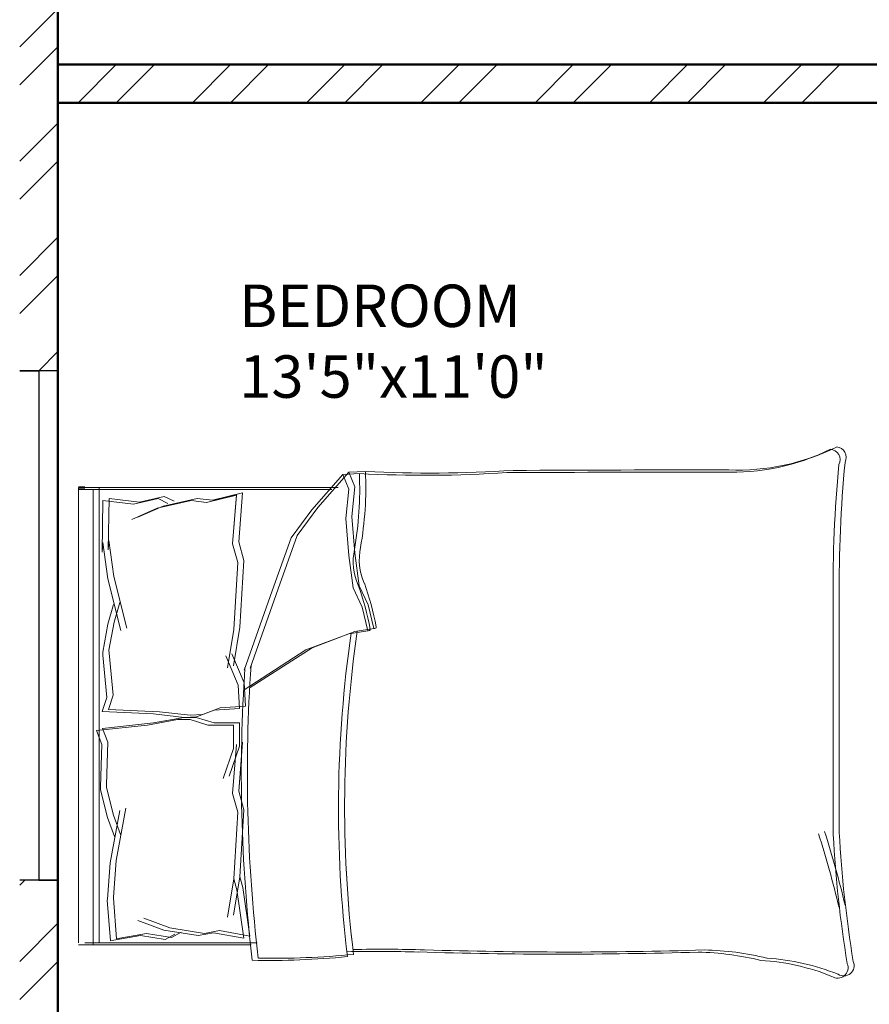
# Model space of a CAD drawing. Units: inches. Extents: x 1901 to 2863, y 888 to 2433.
# Tile 24 of 91: x 2439 to 2540, y 1289 to 1405. Entities that reach past the tile are written whole.
import ezdxf

# ---------------------------------------------------------------- set-up
doc = ezdxf.new("R2010")
doc.units = ezdxf.units.IN
for name, color, linetype, lineweight in [('A-AREA-IDEN', 7, 'Continuous', 18), ('A-FURN', 8, 'Continuous', 18), ('A-GLAZ', 3, 'Continuous', 25), ('A-WALL', 7, 'Continuous', 50), ('A-WALL-PATT', 8, 'Continuous', 13)]:
    doc.layers.add(name, color=color, linetype=linetype, lineweight=lineweight)
doc.styles.get("Standard").update_dxf_attribs({"font": 'arial.ttf'})

# ---------------------------------------------------------------- blocks, each defined once
blk = doc.blocks.new('BED-DOUBLE')
for p, q in [((31.18, 59.32), (27.53, 55.16)), ((31.18, 59.32), (27.53, 55.16)), ((31.9, 59.58), (28.25, 55.42)), ((31.9, 59.58), (28.25, 55.42)), ((33.14, 59.41), (31.18, 59.32, 4.35)), ((33.14, 59.41), (31.18, 59.32, 4.35)), ((31.87, 57.59), (31.18, 59.32)), ((31.87, 57.59), (31.18, 59.32)), ((33.85, 59.67), (31.9, 59.58, 4.35)), ((33.85, 59.67), (31.9, 59.58, 4.35)), ((32.59, 57.85), (31.9, 59.58)), ((32.59, 57.85), (31.9, 59.58)), ((0.03, 57.78), (0.03, 4.12)), ((0.74, 57.78), (30.62, 57.78)), ((0.74, 57.78), (30.62, 57.78)), ((18.63, 56.89), (15.11, 56.01)), ((18.63, 56.88), (15.11, 56.01)), ((19.35, 57.14), (15.83, 56.27)), ((19.35, 57.14), (15.83, 56.27)), ((18.18, 51.12), (18.63, 56.89)), ((18.18, 51.12), (18.63, 56.88)), ((18.9, 51.38), (19.35, 57.14)), ((18.9, 51.38), (19.35, 57.14)), ((31.53, 54.12), (31.87, 57.59)), ((31.53, 54.12), (31.87, 57.59)), ((32.24, 54.37), (32.59, 57.85)), ((32.24, 54.37), (32.59, 57.85)), ((2.9, 56.23), (2.79, 50.16)), ((2.9, 56.23), (2.79, 50.16)), ((2.9, 56.23), (6.5, 55.8)), ((2.9, 56.23), (6.5, 55.8)), ((3.61, 56.48), (3.51, 50.42)), ((3.61, 56.48), (3.51, 50.42)), ((3.61, 56.48), (7.22, 56.06)), ((3.61, 56.48), (7.22, 56.06)), ((6.5, 55.8), (9.39, 56.47)), ((6.5, 55.8), (9.39, 56.47)), ((7.22, 56.06), (10.11, 56.73)), ((7.22, 56.06), (10.11, 56.73)), ((13.31, 56.23), (9.3, 55.33)), ((13.31, 56.23), (9.3, 55.33)), ((9.39, 56.47), (10.56, 55.89)), ((9.39, 56.47), (10.56, 55.89)), ((14.02, 56.48), (10.01, 55.58)), ((14.02, 56.48), (10.01, 55.58)), ((10.11, 56.73), (11.28, 56.15)), ((10.11, 56.73), (11.28, 56.15)), ((15.11, 56.01), (13.31, 56.23)), ((15.11, 56.01), (13.31, 56.23)), ((15.83, 56.27), (14.02, 56.48)), ((15.83, 56.27), (14.02, 56.48)), ((9.3, 55.33), (6.29, 54)), ((9.3, 55.33), (6.29, 54)), ((10.01, 55.58), (7.01, 54.26)), ((10.01, 55.58), (7.01, 54.26)), ((27.53, 55.16), (25.1, 51.86)), ((27.53, 55.16), (25.1, 51.86)), ((28.25, 55.42), (25.81, 52.11)), ((28.25, 55.42), (25.81, 52.11)), ((31.87, 49.77), (31.53, 54.12)), ((31.87, 49.77), (31.53, 54.12)), ((32.59, 50.03), (32.24, 54.37)), ((32.59, 50.03), (32.24, 54.37)), ((2.79, 50.16), (2.88, 51.29)), ((2.79, 50.16), (2.88, 51.29)), ((2.88, 51.29), (3.47, 47.02)), ((2.88, 51.29), (3.47, 47.02)), ((3.51, 50.42), (3.6, 51.54)), ((3.51, 50.42), (3.6, 51.54)), ((3.6, 51.54), (4.19, 47.28)), ((3.6, 51.54), (4.19, 47.28)), ((18.81, 48.92), (18.18, 51.12)), ((18.81, 48.92), (18.18, 51.12)), ((19.52, 49.18), (18.9, 51.38)), ((19.52, 49.18), (18.9, 51.38)), ((25.1, 51.86), (22.84, 45.6)), ((25.1, 51.86), (22.84, 45.6)), ((25.81, 52.11), (23.55, 45.85)), ((25.81, 52.11), (23.55, 45.85)), ((33.11, 46.2), (32.59, 50.03)), ((33.11, 46.2), (32.59, 50.03)), ((18.32, 41.05), (18.81, 48.92)), ((18.32, 41.05), (18.81, 48.92)), ((19.04, 41.31), (19.52, 49.18)), ((19.04, 41.31), (19.52, 49.18)), ((32.39, 45.94), (31.87, 49.77)), ((32.39, 45.94), (31.87, 49.77)), ((3.47, 47.02), (4.99, 40.94)), ((3.47, 47.02), (4.99, 40.94)), ((4.19, 47.28), (5.71, 41.19)), ((4.19, 47.28), (5.71, 41.19)), ((22.84, 45.6), (19.54, 36.24)), ((22.84, 45.6), (19.54, 36.24)), ((23.55, 45.85), (20.26, 36.49)), ((23.55, 45.85), (20.26, 36.49)), ((33.44, 43.68), (32.39, 45.94)), ((33.44, 43.68), (32.39, 45.94)), ((34.15, 43.94), (33.11, 46.2)), ((34.15, 43.94), (33.11, 46.2)), ((4.87, 44.23), (4.2, 41.91)), ((4.87, 44.23), (4.2, 41.91)), ((89, 16.88), (89, 44.51)), ((89, 16.88), (89, 44.51)), ((89.72, 17.13), (89.72, 44.77)), ((89.72, 17.13), (89.72, 44.77)), ((4.15, 43.98), (3.48, 41.66)), ((4.15, 43.98), (3.48, 41.66)), ((34.13, 40.9), (33.44, 43.68)), ((34.13, 40.9), (33.44, 43.68)), ((34.85, 41.16), (34.15, 43.94)), ((34.85, 41.16), (34.15, 43.94)), ((4.2, 41.91), (3.59, 38.62)), ((4.2, 41.91), (3.59, 38.62)), ((3.48, 41.66), (2.87, 38.37)), ((3.48, 41.66), (2.87, 38.37)), ((17.57, 36.53), (18.32, 41.05)), ((17.57, 36.52), (18.32, 41.05)), ((18.29, 36.78), (19.04, 41.31)), ((18.29, 36.78), (19.04, 41.31)), ((27.55, 38.9), (32.59, 40.81)), ((27.55, 38.9), (32.59, 40.81)), ((31.87, 40.55), (34.13, 40.9)), ((31.87, 40.55), (34.13, 40.9)), ((32.59, 40.81), (34.85, 41.16)), ((32.59, 40.81), (34.85, 41.16)), ((26.83, 38.64), (31.87, 40.55)), ((26.83, 38.64), (31.87, 40.55)), ((2.87, 38.37), (2.9, 38.01)), ((2.87, 38.37), (2.9, 38.01)), ((3.59, 38.62), (3.62, 38.26)), ((3.59, 38.62), (3.62, 38.26)), ((19.54, 33.94), (26.83, 38.64)), ((19.54, 33.94), (26.83, 38.64)), ((20.26, 34.19), (27.55, 38.9)), ((20.26, 34.19), (27.55, 38.9)), ((2.9, 38.01), (3.37, 33.03)), ((2.9, 38.01), (3.37, 33.04)), ((3.62, 38.26), (4.09, 33.29)), ((3.62, 38.26), (4.09, 33.29)), ((18.82, 34.49), (17.38, 37.94)), ((18.82, 34.49), (17.38, 37.94)), ((19.54, 34.74), (18.1, 38.19)), ((19.54, 34.74), (18.1, 38.19)), ((18.99, 31.73), (18.82, 34.49)), ((18.99, 31.73), (18.82, 34.49)), ((19.71, 31.99), (19.54, 34.74)), ((19.71, 31.99), (19.54, 34.74)), ((3.37, 33.04), (2.82, 31.37)), ((3.37, 33.03), (2.82, 31.37)), ((4.09, 33.29), (3.54, 31.63)), ((4.09, 33.29), (3.54, 31.63)), ((2.82, 31.37), (8.86, 31.1)), ((2.82, 31.37), (8.86, 31.1)), ((3.54, 31.63), (9.58, 31.36)), ((3.54, 31.63), (9.58, 31.36)), ((9.58, 31.36), (13.18, 30.93)), ((9.58, 31.36), (13.18, 30.93)), ((13.92, 30.77), (15.99, 31.55)), ((13.92, 30.77), (15.99, 31.55)), ((14.64, 31.02), (16.71, 31.8)), ((14.64, 31.02), (16.71, 31.8)), ((15.99, 31.55), (18.99, 31.73)), ((15.99, 31.55), (18.99, 31.73)), ((16.71, 31.8), (19.71, 31.99)), ((16.71, 31.8), (19.71, 31.99)), ((8.13, 29.78), (11.7, 30.43)), ((8.13, 29.78), (11.7, 30.43)), ((8.85, 30.04), (12.42, 30.69)), ((8.85, 30.04), (12.42, 30.69)), ((8.86, 31.1), (12.46, 30.68)), ((8.86, 31.1), (12.46, 30.68)), ((11.7, 30.43), (13.16, 30.43)), ((11.7, 30.43), (13.16, 30.43)), ((12.42, 30.69), (13.88, 30.69)), ((12.42, 30.69), (13.88, 30.69)), ((12.46, 30.68), (13.92, 30.77)), ((12.46, 30.68), (13.92, 30.77)), ((13.16, 30.43), (15.28, 29.78)), ((13.16, 30.43), (15.28, 29.78)), ((13.18, 30.93), (14.64, 31.02)), ((13.18, 30.93), (14.64, 31.02)), ((13.88, 30.69), (15.99, 30.04)), ((13.88, 30.69), (15.99, 30.04)), ((2.13, 29.14), (8.13, 29.78)), ((2.13, 29.14), (8.13, 29.78)), ((2.78, 27.51), (2.13, 29.14)), ((2.78, 27.51), (2.13, 29.14)), ((2.84, 29.39), (8.85, 30.04)), ((2.84, 29.39), (8.85, 30.04)), ((3.49, 27.77), (2.84, 29.39)), ((3.49, 27.77), (2.84, 29.39)), ((15.28, 29.78), (18.29, 29.78)), ((15.28, 29.78), (18.29, 29.78)), ((15.99, 30.04), (19, 30.04)), ((15.99, 30.04), (19, 30.04)), ((18.29, 29.78), (18.29, 27.03)), ((18.29, 29.78), (18.29, 27.03)), ((19, 30.04), (19, 27.28)), ((19, 30.04), (19, 27.28)), ((2.61, 22.52), (2.78, 27.51)), ((2.61, 22.52), (2.78, 27.51)), ((3.33, 22.78), (3.49, 27.77)), ((3.33, 22.78), (3.49, 27.77)), ((18.29, 27.03), (17.06, 23.49)), ((18.29, 27.03), (17.06, 23.5)), ((19, 27.28), (17.78, 23.75)), ((19, 27.28), (17.78, 23.75)), ((18.18, 21.73), (18.63, 27.49)), ((18.18, 21.73), (18.63, 27.49)), ((18.9, 21.98), (19.35, 27.75)), ((18.9, 21.98), (19.35, 27.74)), ((2.61, 22.16), (2.61, 22.52)), ((2.61, 22.16), (2.61, 22.52)), ((3.42, 18.91), (2.61, 22.16)), ((3.42, 18.91), (2.61, 22.16)), ((3.33, 22.42), (3.33, 22.78)), ((3.33, 22.42), (3.33, 22.78)), ((4.14, 19.17), (3.33, 22.42)), ((4.14, 19.17), (3.33, 22.42)), ((18.81, 19.53), (18.18, 21.73)), ((18.81, 19.53), (18.18, 21.73)), ((19.52, 19.78), (18.9, 21.98)), ((19.52, 19.78), (18.9, 21.98)), ((3.75, 13.56), (4.89, 19.73)), ((3.75, 13.56), (4.89, 19.73)), ((4.47, 13.81), (5.6, 19.98)), ((4.47, 13.81), (5.6, 19.98)), ((19.04, 11.91), (19.52, 19.78)), ((19.04, 11.91), (19.52, 19.78)), ((4.24, 16.64), (3.42, 18.91)), ((4.24, 16.64), (3.42, 18.91)), ((4.95, 16.9), (4.14, 19.17)), ((4.95, 16.9), (4.14, 19.17)), ((18.32, 11.66), (18.81, 19.53)), ((18.32, 11.66), (18.81, 19.53)), ((3.42, 9.27), (3.75, 13.56)), ((3.42, 9.27), (3.75, 13.56)), ((4.14, 9.52), (4.47, 13.81)), ((4.14, 9.52), (4.47, 13.81)), ((17.57, 7.13), (18.32, 11.66)), ((17.57, 7.13), (18.32, 11.66)), ((18.29, 7.38), (19.04, 11.91)), ((18.29, 7.39), (19.04, 11.91)), ((18.32, 11.66), (18.68, 10.38)), ((18.32, 11.66), (18.68, 10.38)), ((19.04, 11.91), (19.4, 10.64)), ((19.04, 11.91), (19.4, 10.64)), ((19.4, 10.64), (20.21, 4.92)), ((19.4, 10.64), (20.21, 4.92)), ((4.12, 9.4), (4.14, 9.52)), ((4.12, 9.4), (4.14, 9.52)), ((4.49, 4.6), (4.12, 9.4)), ((4.49, 4.6), (4.12, 9.4)), ((18.68, 10.38), (19.5, 4.66)), ((18.68, 10.38), (19.5, 4.66)), ((3.4, 9.15), (3.42, 9.27)), ((3.4, 9.15), (3.42, 9.27)), ((3.77, 4.34), (3.4, 9.15)), ((3.77, 4.34), (3.4, 9.15)), ((10.8, 5.89), (7.71, 7.03)), ((10.8, 5.89), (7.71, 7.03)), ((10.08, 5.63), (7, 6.77)), ((10.08, 5.63), (7, 6.77)), ((14.86, 5.24), (10.8, 5.89)), ((14.86, 5.24), (10.8, 5.89)), ((3.75, 4.34), (7.32, 4.99)), ((3.75, 4.34), (7.32, 4.99)), ((4.47, 4.59), (8.04, 5.24)), ((4.47, 4.59), (8.04, 5.24)), ((7.32, 4.99), (10.24, 4.5)), ((7.32, 4.99), (10.24, 4.5)), ((8.04, 5.24), (10.96, 4.75)), ((8.04, 5.24), (10.96, 4.76)), ((14.14, 4.99), (10.08, 5.63)), ((14.14, 4.99), (10.08, 5.63)), ((10.24, 4.5), (11.38, 5.15)), ((10.24, 4.5), (11.38, 5.15)), ((10.96, 4.76), (12.1, 5.4)), ((10.96, 4.75), (12.1, 5.4)), ((15.92, 5.31), (14.14, 4.99)), ((15.92, 5.31), (14.14, 4.99)), ((16.64, 5.57), (14.86, 5.24)), ((16.64, 5.57), (14.86, 5.24)), ((19.5, 4.66), (15.92, 5.31)), ((19.5, 4.66), (15.92, 5.31)), ((20.21, 4.92), (16.64, 5.57)), ((20.21, 4.92), (16.64, 5.57))]:
    blk.add_line(p, q)
for centre, radius, start, end in [((77.12, 85.47), 25.9, 267.4714, 296.4681), ((77.12, 85.47), 25.9, 267.4714, 296.4681), ((77.84, 85.73), 25.9, 267.4714, 296.4681), ((77.84, 85.73), 25.9, 267.4714, 296.4681), ((88.58, 61.05), 1.24, 332.6588, 86.02), ((88.58, 61.05), 1.24, 332.6588, 86.02), ((89.3, 61.31), 1.24, 332.6588, 86.02), ((89.3, 61.31), 1.24, 332.6588, 86.02), ((238.36, 46.17), 149.37, 174.4998, 180.6351), ((238.36, 46.17), 149.37, 174.4998, 180.6351), ((239.08, 46.42), 149.37, 174.4998, 180.6351), ((239.08, 46.42), 149.37, 174.4998, 180.6351), ((-7.45, 57.59), 40.62, 349.8763, 2.5657), ((-7.45, 57.59), 40.62, 349.8763, 2.5657), ((40.8, 204.6), 145.39, 266.9791, 273.8365), ((40.8, 204.6), 145.39, 266.9791, 273.8365), ((-6.73, 57.85), 40.62, 349.8763, 2.5657), ((-6.73, 57.85), 40.62, 349.8763, 2.5657), ((41.52, 204.86), 145.39, 266.9791, 273.8365), ((41.52, 204.86), 145.39, 266.9791, 273.8365), ((76.17, -5062.23), 5121.82, 90.00217, 90.28689), ((76.17, -5062.23), 5121.82, 90.00217, 90.28689), ((76.89, -5061.97), 5121.82, 90.00217, 90.28689), ((76.89, -5061.97), 5121.82, 90.00217, 90.28689), ((39.4, 49.08), 6.99, 168.6608, 203.7384), ((39.4, 49.08), 6.99, 168.6608, 203.7384), ((40.11, 49.33), 6.99, 168.6608, 203.7384), ((40.11, 49.33), 6.99, 168.6608, 203.7384), ((2.41, 35.2), 33.29, 10.6617, 19.8806), ((2.41, 35.2), 33.29, 10.6617, 19.8806), ((1.69, 34.94), 33.29, 10.6617, 19.8806), ((1.69, 34.94), 33.29, 10.6617, 19.8806), ((176.25, 20.16), 144.86, 171.7845, 186.9006), ((176.25, 20.15), 144.86, 171.7845, 186.9006), ((34.2, 41.1), 0.207, 250.2464, 1.1377), ((34.2, 41.1), 0.207, 250.2464, 1.1377), ((34.92, 41.35), 0.207, 250.2464, 1.1377), ((34.92, 41.35), 0.207, 250.2464, 1.1377), ((175.53, 19.9), 144.86, 171.7845, 186.9006), ((175.53, 19.9), 144.86, 171.7845, 186.9006), ((204.43, 23.94), 185.22, 176.0865, 186.7821), ((204.43, 23.94), 185.22, 176.0865, 186.7821), ((205.14, 24.2), 185.22, 176.0865, 186.7821), ((205.14, 24.2), 185.22, 176.0865, 186.7821), ((225.52, 24.02), 136.7, 182.9958, 189.4091), ((225.52, 24.02), 136.7, 182.9958, 189.4091), ((226.23, 24.28), 136.7, 182.9958, 189.4091), ((226.23, 24.28), 136.7, 182.9958, 189.4091), ((22.59, 95.58), 93.53, 268.7218, 275.604), ((22.59, 95.58), 93.53, 268.7218, 275.604), ((23.31, 95.84), 93.53, 268.7218, 275.604), ((23.31, 95.84), 93.53, 268.7218, 275.604), ((35.03, -187.88), 190.99, 88.4762, 91.0082), ((35.03, -187.88), 190.99, 88.4762, 91.0082), ((35.74, -187.62), 190.99, 88.4762, 91.0082), ((35.74, -187.62), 190.99, 88.4762, 91.0082), ((56.85, 544.3), 541.51, 268.2277, 271.7185), ((56.85, 544.3), 541.51, 268.2277, 271.7185), ((57.57, 544.55), 541.51, 268.2277, 271.7185), ((57.57, 544.55), 541.51, 268.2277, 271.7185), ((72.46, -30.24), 33.27, 76.0648, 88.9113), ((72.46, -30.24), 33.27, 76.0648, 88.9113), ((73.18, -29.98), 33.27, 76.0648, 88.9113), ((73.18, -29.98), 33.27, 76.0648, 88.9113), ((78.93, -24.35), 26.45, 67.9751, 86.652), ((78.93, -24.35), 26.45, 67.9751, 86.652), ((79.65, -24.1), 26.45, 67.9751, 86.652), ((79.65, -24.1), 26.45, 67.9751, 86.652), ((89.53, 1.18), 1.22, 236.1736, 23.4781), ((89.53, 1.18), 1.22, 236.1736, 23.4781), ((90.25, 1.44), 1.22, 236.1736, 23.4781), ((90.25, 1.44), 1.22, 236.1736, 23.4781)]:
    blk.add_arc(centre, radius, start, end)
blk = doc.blocks.new('WIN-60')
for p, q in [((0, 4.5), (0, 0)), ((60, 2.25), (60, 4.5)), ((60, 4.5), (60, 0)), ((0, 0), (0, 2.25)), ((0, 2.25), (60, 2.25))]:
    blk.add_line(p, q)

msp = doc.modelspace()

# ---------------------------------------------------------------- hatches: boundary and pattern name
at = {"layer": 'A-WALL-PATT'}
h = msp.add_hatch(dxfattribs=at)
h.set_pattern_fill('ANSI32', color=256)
h.paths.add_polyline_path([(2192.5, 2274.13), (2141.26, 2274.13), (2141.26, 2269.63), (2192.5, 2269.63)])
h.paths.add_polyline_path([(2259.93, 2274.13), (2216.5, 2274.13), (2216.5, 2269.63), (2255.43, 2269.63), (2255.43, 2214.63), (2250.81, 2214.63), (2250.81, 2210.13), (2259.93, 2210.13), (2259.93, 2215.13), (2271.76, 2215.13), (2271.76, 2217.38), (2271.76, 2219.63), (2259.93, 2219.63)])
h.paths.add_polyline_path([(2171.43, 2269.63), (2166.93, 2269.63), (2166.93, 2219.63), (2121.24, 2219.63), (2121.24, 2215.13), (2166.93, 2215.13), (2166.93, 2083.13), (2161.81, 2083.13), (2161.81, 2078.63), (2171.43, 2078.63), (2177, 2078.63), (2177, 2080.88), (2177, 2083.13), (2171.43, 2083.13), (2171.43, 2210.13), (2230.91, 2210.13), (2230.91, 2212.38), (2230.91, 2214.63), (2171.43, 2214.63)])
h.paths.add_polyline_path([(2117.26, 2274.13), (2089.43, 2274.13), (2089.43, 2219.63), (2081.14, 2219.63), (2081.14, 2215.13), (2089.43, 2215.13), (2098, 2215.13), (2098, 2217.38), (2098, 2219.63), (2093.93, 2219.63), (2093.93, 2269.63), (2117.26, 2269.63), (2117.26, 2271.88)])
h.paths.add_polyline_path([(2343.43, 2219.63), (2329.29, 2219.63), (2329.29, 2215.13), (2338.93, 2215.13), (2338.93, 2184.74), (2343.43, 2184.74)])
h.paths.add_polyline_path([(2338.93, 2083.13), (2329.29, 2083.13), (2208.97, 2083.13), (2208.97, 2078.63), (2338.93, 2078.63)])
h.paths.add_polyline_path([(2343.43, 2136.74), (2338.93, 2136.74), (2338.93, 1872.63), (2343.43, 1872.63)])
h.paths.add_polyline_path([(2343.43, 1863.63), (2397.68, 1863.63), (2397.68, 1821.63), (2384.14, 1821.63), (2384.14, 1812.63), (2418.33, 1812.63), (2418.33, 1817.13), (2418.33, 1821.63), (2406.68, 1821.63), (2406.68, 1863.63), (2459.5, 1863.63), (2459.5, 1821.63), (2447.14, 1821.63), (2447.14, 1812.63), (2459.5, 1812.63), (2468.5, 1812.63), (2468.5, 1872.63), (2394.43, 1872.63), (2334.43, 1872.63), (2334.43, 1812.63), (2343.43, 1812.63), (2353.25, 1812.63), (2353.25, 1821.63), (2343.43, 1821.63)])
h.paths.add_polyline_path([(2510.01, 1872.63), (2468.5, 1872.63), (2468.5, 1868.13), (2510.01, 1868.13)])
h.paths.add_polyline_path([(2514.01, 1817.13), (2468.5, 1817.13), (2468.5, 1812.63), (2482.11, 1812.63), (2482.11, 1800.61), (2486.61, 1800.61), (2486.61, 1812.63), (2514.01, 1812.63)])
h.paths.add_polyline_path([(2299.25, 1814.88), (2299.25, 1817.13), (2295.93, 1817.13), (2295.93, 1854.17), (2293.68, 1854.17), (2291.43, 1854.17), (2291.43, 1817.13), (2266.11, 1817.13), (2266.11, 1812.63), (2299.25, 1812.63)])
h.paths.add_polyline_path([(2218.11, 1817.13), (2206.46, 1817.13), (2171.43, 1817.13), (2171.43, 1949.13), (2190.1, 1949.13), (2190.1, 1953.63), (2163.47, 1953.63), (2163.47, 1949.13), (2166.93, 1949.13), (2166.93, 1817.13), (2114.3, 1817.13), (2114.3, 1812.63), (2218.11, 1812.63)])
h.paths.add_polyline_path([(2029.43, 1970.92), (2024.93, 1970.92), (2024.93, 1912.72), (2029.43, 1912.72)])
h.paths.add_polyline_path([(2132.3, 1953.63), (2113.93, 1953.63), (2113.93, 1975.89), (2111.68, 1975.89), (2109.43, 1975.89), (2109.43, 1953.63), (2029.43, 1953.63), (2029.43, 1949.13), (2132.3, 1949.13)])
h.paths.add_polyline_path([(2029.43, 1853.61), (2029.31, 1853.61), (2029.31, 1853.61), (2029.43, 1853.61), (2029.43, 1864.72), (2024.93, 1864.72), (2024.93, 1812.63), (2066.3, 1812.63), (2066.3, 1814.88), (2066.3, 1817.13), (2029.43, 1817.13)])
h.paths.add_polyline_path([(2122.93, 2010.09), (2120.68, 2010.09), (2118.43, 2010.09), (2118.43, 2006.13), (2029.43, 2006.13), (2029.43, 2001.63), (2109.43, 2001.63), (2109.43, 1998.04), (2113.93, 1998.04), (2113.93, 2001.63), (2122.93, 2001.63)])
h.paths.add_polyline_path([(2029.43, 2031.38), (2024.93, 2031.38), (2024.93, 1994.92), (2027.18, 1994.92), (2029.43, 1994.92)])
h.paths.add_polyline_path([(2029.43, 2136.74), (2024.93, 2136.74), (2024.93, 2067.38), (2027.18, 2067.38), (2029.43, 2067.38)])
h.paths.add_polyline_path([(2125.62, 2083.13), (2029.43, 2083.13), (2029.43, 2078.63), (2118.43, 2078.63), (2118.43, 2030.71), (2122.93, 2030.71), (2122.93, 2078.63), (2125.62, 2078.63)])
h.paths.add_polyline_path([(2029.43, 2215.13), (2040.47, 2215.13), (2040.47, 2217.38), (2040.47, 2219.63), (2024.93, 2219.63), (2024.93, 2184.74), (2029.43, 2184.74), (2029.43, 2187.78)])
h.paths.add_polyline_path([(2686.43, 2274.13), (2659.28, 2274.13), (2659.28, 2269.63), (2681.93, 2269.63), (2681.93, 2219.63), (2676.82, 2219.63), (2676.82, 2215.13), (2681.93, 2215.13), (2697.01, 2215.13), (2697.01, 2217.38), (2697.01, 2219.63), (2686.43, 2219.63)])
h.paths.add_polyline_path([(2609.93, 2269.63), (2635.28, 2269.63), (2635.28, 2274.13), (2571.43, 2274.13), (2571.43, 2269.63), (2605.43, 2269.63), (2605.43, 2214.63), (2549.1, 2214.63), (2549.1, 2210.13), (2605.43, 2210.13), (2605.43, 2083.13), (2601.01, 2083.13), (2601.01, 2080.88), (2601.01, 2078.63), (2609.93, 2078.63), (2616.16, 2078.63), (2616.16, 2080.88), (2616.16, 2083.13), (2609.93, 2083.13), (2609.93, 2215.13), (2651.46, 2215.13), (2651.46, 2217.38), (2651.46, 2219.63), (2609.93, 2219.63)])
h.paths.add_polyline_path([(2521.43, 2269.63), (2547.43, 2269.63), (2547.43, 2271.88), (2547.43, 2274.13), (2516.93, 2274.13), (2516.93, 2219.63), (2506.41, 2219.63), (2506.41, 2215.13), (2516.93, 2215.13), (2516.93, 2210.13), (2525.4, 2210.13), (2525.4, 2212.38), (2525.4, 2214.63), (2521.43, 2214.63)])
h.paths.add_polyline_path([(2456.01, 2219.63), (2439.43, 2219.63), (2439.43, 2187.89), (2443.93, 2187.89), (2443.93, 2215.13), (2456.01, 2215.13)])
h.paths.add_polyline_path([(2752.93, 2219.63), (2739.48, 2219.63), (2739.48, 2215.13), (2748.43, 2215.13), (2748.43, 2187.89), (2752.93, 2187.89)])
h.paths.add_polyline_path([(2752.93, 2139.89), (2748.43, 2139.89), (2748.43, 2083.13), (2648.42, 2083.13), (2648.42, 2078.63), (2654.93, 2078.63), (2654.93, 2039.44), (2659.43, 2039.44), (2659.43, 2078.63), (2748.43, 2078.63), (2748.43, 2063.43), (2752.93, 2063.43)])
h.paths.add_polyline_path([(2752.93, 2010.63), (2659.43, 2010.63), (2659.43, 2015.65), (2654.93, 2015.65), (2654.93, 2010.63), (2605.43, 2010.63), (2605.43, 1920.97), (2609.93, 1920.97), (2609.93, 2006.13), (2748.43, 2006.13), (2748.43, 1982.47), (2752.93, 1982.47)])
h.paths.add_polyline_path([(2752.93, 2027.43), (2748.43, 2027.43), (2748.43, 2010.63), (2752.93, 2010.63)])
h.paths.add_polyline_path([(2748.43, 1886.13), (2609.93, 1886.13), (2609.93, 1889.72), (2605.43, 1889.72), (2605.43, 1861.26), (2609.93, 1861.26), (2609.93, 1881.63), (2748.43, 1881.63)])
h.paths.add_polyline_path([(2456.86, 2228.83), (2498.4, 2228.83), (2498.4, 2247.49), (2456.86, 2247.49)], flags=9)
h.paths.add_polyline_path([(2038.6, 2237.42), (2080.17, 2237.42), (2080.17, 2256.08), (2038.6, 2256.08)], flags=9)
h.paths.add_polyline_path([(2292.01, 1062.39), (2539.93, 1062.39), (2539.93, 1099.49), (2292.01, 1099.49)], flags=9)
h.paths.add_polyline_path([(2424.91, 1832.25), (2448.51, 1832.25), (2448.51, 1846.68), (2424.91, 1846.68)], flags=25)
h.paths.add_polyline_path([(2359.08, 1832.25), (2382.68, 1832.25), (2382.68, 1846.68), (2359.08, 1846.68)], flags=25)
h.paths.add_polyline_path([(2352.9, 1684.8), (2367.54, 1684.8), (2367.54, 1697.17), (2352.9, 1697.17)], flags=9)
h.paths.add_polyline_path([(2079.29, 1755.83), (2169.02, 1755.83), (2169.02, 1774.37), (2079.29, 1774.37)], flags=9)
h.paths.add_polyline_path([(2404.09, 1373.86), (2404.09, 1463.59), (2385.54, 1463.59), (2385.54, 1373.86)], flags=9)
h.paths.add_polyline_path([(2268.09, 2236.37), (2309.64, 2236.37), (2309.64, 2255.03), (2268.09, 2255.03)], flags=9)
h.paths.add_polyline_path([(2575.96, 1700.95), (2665.7, 1700.95), (2665.7, 1719.5), (2575.96, 1719.5)], flags=9)
h.paths.add_polyline_path([(2302.96, 1878.47), (2329.52, 1878.47), (2329.52, 1888.78), (2302.96, 1888.78)], flags=9)
h.paths.add_polyline_path([(2097.42, 2240.58), (2126.57, 2240.58), (2126.57, 2259.23), (2097.42, 2259.23)], flags=9)
h.paths.add_polyline_path([(2208.72, 2246.12), (2237.88, 2246.12), (2237.88, 2264.78), (2208.72, 2264.78)], flags=9)
h.paths.add_polyline_path([(2038.15, 1925.96), (2076.99, 1925.96), (2076.99, 1944.62), (2038.15, 1944.62)], flags=9)
h.paths.add_polyline_path([(2239.14, 1926.67), (2288.46, 1926.67), (2288.46, 1945.33), (2239.14, 1945.33)], flags=9)
h.paths.add_polyline_path([(2175.43, 2007.33), (2212.36, 2007.33), (2212.36, 2025.99), (2175.43, 2025.99)], flags=9)
h.paths.add_polyline_path([(2225.03, 2091.79), (2263.87, 2091.79), (2263.87, 2110.45), (2225.03, 2110.45)], flags=9)
h.paths.add_polyline_path([(2035.4, 2098.48), (2074.24, 2098.48), (2074.24, 2117.14), (2035.4, 2117.14)], flags=9)
h.paths.add_polyline_path([(2050.1, 2029.21), (2083.26, 2029.21), (2083.26, 2047.87), (2050.1, 2047.87)], flags=9)
h.paths.add_polyline_path([(2069.68, 1956.72), (2098.83, 1956.72), (2098.83, 1975.38), (2069.68, 1975.38)], flags=25)
h.paths.add_polyline_path([(2328.62, 1753.34), (2361.66, 1753.34), (2361.66, 1771.99), (2328.62, 1771.99)], flags=9)
h.paths.add_polyline_path([(2395.16, 2060.89), (2395.16, 2140.65), (2378.68, 2140.65), (2378.68, 2060.89)], flags=9)
h.paths.add_polyline_path([(2463.73, 2059.02), (2492.89, 2059.02), (2492.89, 2077.68), (2463.73, 2077.68)], flags=9)
h.paths.add_polyline_path([(2458.03, 2181.54), (2496.87, 2181.54), (2496.87, 2200.19), (2458.03, 2200.19)], flags=9)
h.paths.add_polyline_path([(2527.58, 2243.07), (2556.73, 2243.07), (2556.73, 2261.73), (2527.58, 2261.73)], flags=9)
h.paths.add_polyline_path([(2694.46, 2232.77), (2736.03, 2232.77), (2736.03, 2251.42), (2694.46, 2251.42)], flags=9)
h.paths.add_polyline_path([(2637.82, 2249.22), (2666.98, 2249.22), (2666.98, 2267.88), (2637.82, 2267.88)], flags=9)
h.paths.add_polyline_path([(2623.69, 2183.54), (2662.53, 2183.54), (2662.53, 2202.2), (2623.69, 2202.2)], flags=9)
h.paths.add_polyline_path([(2691.97, 2021.5), (2725.12, 2021.5), (2725.12, 2040.16), (2691.97, 2040.16)], flags=9)
h.paths.add_polyline_path([(2621.04, 1975.91), (2662.34, 1975.91), (2662.34, 1994.57), (2621.04, 1994.57)], flags=25)
h.paths.add_polyline_path([(2479.03, 1927.62), (2519.84, 1927.62), (2519.84, 1946.28), (2479.03, 1946.28)], flags=9)
h.paths.add_polyline_path([(2670.94, 1849.08), (2716.01, 1849.08), (2716.01, 1867.73), (2670.94, 1867.73)], flags=9)
h.paths.add_polyline_path([(2523.61, 1782.96), (2550.17, 1782.96), (2550.17, 1793.26), (2523.61, 1793.26)], flags=9)
h.paths.add_polyline_path([(2450.84, 1207.33), (2492.39, 1207.33), (2492.39, 1225.99), (2450.84, 1225.99)], flags=9)
h.paths.add_polyline_path([(2527.75, 1203.84), (2556.91, 1203.84), (2556.91, 1222.5), (2527.75, 1222.5)], flags=9)
h.paths.add_polyline_path([(2639.11, 1207.2), (2668.27, 1207.2), (2668.27, 1225.86), (2639.11, 1225.86)], flags=9)
h.paths.add_polyline_path([(2692.59, 1218.97), (2734.17, 1218.97), (2734.17, 1237.62), (2692.59, 1237.62)], flags=9)
h.paths.add_polyline_path([(2669.27, 1366.33), (2708.11, 1366.33), (2708.11, 1384.99), (2669.27, 1384.99)], flags=9)
h.paths.add_polyline_path([(2463.31, 1358.03), (2502.15, 1358.03), (2502.15, 1376.69), (2463.31, 1376.69)], flags=9)
h.paths.add_polyline_path([(2494.72, 1449.96), (2531.65, 1449.96), (2531.65, 1468.62), (2494.72, 1468.62)], flags=9)
h.paths.add_polyline_path([(2675.57, 1422.16), (2708.72, 1422.16), (2708.72, 1440.81), (2675.57, 1440.81)], flags=9)
h.paths.add_polyline_path([(2685.63, 1493.89), (2714.79, 1493.89), (2714.79, 1512.55), (2685.63, 1512.55)], flags=9)
h.paths.add_polyline_path([(2686.8, 1529.91), (2725.65, 1529.91), (2725.65, 1548.57), (2686.8, 1548.57)], flags=9)
h.paths.add_polyline_path([(2503.65, 1537.99), (2552.97, 1537.99), (2552.97, 1556.65), (2503.65, 1556.65)], flags=9)
h.paths.add_polyline_path([(2291.71, 1643.5), (2318.28, 1643.5), (2318.28, 1653.81), (2291.71, 1653.81)], flags=9)
h.paths.add_polyline_path([(2450.63, 1610.52), (2477.19, 1610.52), (2477.19, 1620.82), (2450.63, 1620.82)], flags=9)
h.paths.add_polyline_path([(2359.99, 1551.81), (2422.25, 1551.81), (2422.25, 1562.12), (2359.99, 1562.12)], flags=9)
h.paths.add_polyline_path([(2280.11, 1249.01), (2321.65, 1249.01), (2321.65, 1267.66), (2280.11, 1267.66)], flags=9)
h.paths.add_polyline_path([(2164.06, 1274.23), (2193.22, 1274.23), (2193.22, 1292.89), (2164.06, 1292.89)], flags=9)
h.paths.add_polyline_path([(2118.21, 1277.69), (2151.25, 1277.69), (2151.25, 1296.35), (2118.21, 1296.35)], flags=9)
h.paths.add_polyline_path([(2031.95, 1268.53), (2073.52, 1268.53), (2073.52, 1287.19), (2031.95, 1287.19)], flags=9)
h.paths.add_polyline_path([(2050.2, 1409.08), (2089.04, 1409.08), (2089.04, 1427.74), (2050.2, 1427.74)], flags=9)
h.paths.add_polyline_path([(2243.74, 1421.03), (2282.58, 1421.03), (2282.58, 1439.69), (2243.74, 1439.69)], flags=9)
h.paths.add_polyline_path([(2190.75, 1509.77), (2231.56, 1509.77), (2231.56, 1528.43), (2190.75, 1528.43)], flags=9)
h.paths.add_polyline_path([(2058.39, 1475.42), (2091.55, 1475.42), (2091.55, 1494.07), (2058.39, 1494.07)], flags=9)
h.paths.add_polyline_path([(2062.45, 1553.09), (2091.6, 1553.09), (2091.6, 1571.75), (2062.45, 1571.75)], flags=9)
h.paths.add_polyline_path([(2219.52, 1590.37), (2266.15, 1590.37), (2266.15, 1609.02), (2219.52, 1609.02)], flags=9)
h.paths.add_polyline_path([(2041.07, 1584.19), (2079.91, 1584.19), (2079.91, 1602.85), (2041.07, 1602.85)], flags=9)
h = msp.add_hatch(dxfattribs=at)
h.set_pattern_fill('ANSI32', color=256)
h.paths.add_polyline_path([(2443.93, 2139.89), (2439.43, 2139.89), (2439.43, 2069.35), (2441.68, 2069.35), (2443.93, 2069.35), (2443.93, 2078.63), (2521.93, 2078.63), (2521.93, 2075.07), (2524.18, 2075.07), (2526.43, 2075.07), (2526.43, 2078.63), (2571.75, 2078.63), (2571.75, 2080.88), (2571.75, 2083.13), (2443.93, 2083.13)])
h.paths.add_polyline_path([(2526.43, 2054.63), (2524.18, 2054.63), (2521.93, 2054.63), (2521.93, 2030.63), (2443.93, 2030.63), (2443.93, 2045.35), (2439.43, 2045.35), (2439.43, 1983.87), (2443.93, 1983.87), (2443.93, 2026.13), (2521.93, 2026.13), (2526.43, 2026.13)])
h.paths.add_polyline_path([(2443.93, 1923.87), (2439.43, 1923.87), (2439.43, 1872.63), (2443.93, 1872.63)])
h.paths.add_polyline_path([(2636.23, 1766.13), (2609.93, 1766.13), (2609.93, 1779.79), (2605.43, 1779.79), (2605.43, 1766.13), (2486.61, 1766.13), (2486.61, 1770.67), (2482.11, 1770.67), (2482.11, 1766.13), (2482.11, 1761.63), (2636.23, 1761.63), (2636.23, 1763.88)])
h.paths.add_polyline_path([(2519.54, 1663.38), (2519.54, 1665.63), (2494.93, 1665.63), (2481.83, 1665.63), (2481.83, 1663.38), (2481.83, 1661.13), (2490.43, 1661.13), (2490.43, 1640.16), (2494.93, 1640.16), (2494.93, 1661.13), (2519.54, 1661.13)])
h.paths.add_polyline_path([(2443.93, 1712.13), (2443.93, 1716.63), (2414.46, 1716.63), (2414.46, 1712.13), (2439.43, 1712.13), (2439.43, 1545.51), (2443.93, 1545.51), (2443.93, 1661.13), (2448.47, 1661.13), (2448.47, 1665.63), (2443.93, 1665.63)])
h.paths.add_polyline_path([(2343.43, 1712.13), (2365.52, 1712.13), (2365.52, 1714.38), (2365.52, 1716.63), (2333.87, 1716.63), (2333.87, 1714.38), (2333.87, 1712.13), (2338.93, 1712.13), (2338.93, 1575.63), (2338.93, 1545.51), (2343.43, 1545.51), (2343.43, 1547.51), (2343.43, 1580.13)])
h.paths.add_polyline_path([(2752.93, 1665.63), (2579.54, 1665.63), (2579.54, 1661.13), (2615.93, 1661.13), (2615.93, 1529.13), (2598.93, 1529.13), (2598.93, 1524.63), (2623.13, 1524.63), (2623.13, 1526.88), (2623.13, 1529.13), (2620.43, 1529.13), (2620.43, 1661.13), (2748.43, 1661.13), (2748.43, 1633.5), (2752.93, 1633.5)])
h.paths.add_polyline_path([(2752.93, 1419.93), (2748.43, 1419.93), (2748.43, 1400.13), (2659.43, 1400.13), (2659.43, 1444.33), (2657.18, 1444.33), (2654.93, 1444.33), (2654.93, 1400.13), (2643.65, 1400.13), (2643.65, 1395.63), (2748.43, 1395.63), (2748.43, 1364.04), (2752.93, 1364.04)])
h.paths.add_polyline_path([(2752.93, 1492.88), (2748.43, 1492.88), (2748.43, 1476.63), (2667.43, 1476.63), (2667.43, 1479.71), (2665.18, 1479.71), (2662.93, 1479.71), (2662.93, 1476.63), (2654.93, 1476.63), (2654.93, 1469.54), (2659.43, 1469.54), (2659.43, 1472.13), (2748.43, 1472.13), (2748.43, 1455.93), (2752.93, 1455.93)])
h.paths.add_polyline_path([(2752.93, 1304.04), (2748.43, 1304.04), (2748.43, 1263.63), (2738.66, 1263.63), (2738.66, 1259.13), (2752.93, 1259.13)])
h.paths.add_polyline_path([(2685.93, 1259.13), (2695.49, 1259.13), (2695.49, 1261.38), (2695.49, 1263.63), (2677.84, 1263.63), (2677.84, 1261.38), (2677.84, 1259.13), (2681.43, 1259.13), (2681.43, 1203.63), (2653.28, 1203.63), (2653.28, 1199.13), (2685.93, 1199.13), (2685.93, 1203.63)])
h.paths.add_polyline_path([(2609.43, 1395.63), (2611.85, 1395.63), (2611.85, 1400.13), (2598.89, 1400.13), (2598.89, 1397.88), (2598.89, 1395.63), (2604.93, 1395.63), (2604.93, 1268.13), (2554.73, 1268.13), (2554.73, 1265.88), (2554.73, 1263.63), (2604.93, 1263.63), (2604.93, 1203.63), (2571.31, 1203.63), (2571.31, 1199.13), (2604.93, 1199.13), (2629.28, 1199.13), (2629.28, 1201.38), (2629.28, 1203.63), (2609.43, 1203.63), (2609.43, 1258.63), (2609.43, 1259.13), (2654.8, 1259.13), (2654.8, 1263.63), (2609.43, 1263.63)])
h.paths.add_polyline_path([(2443.93, 1304.04), (2439.43, 1304.04), (2439.43, 1259.13), (2443.93, 1259.13), (2456.16, 1259.13), (2456.16, 1261.38), (2456.16, 1263.63), (2443.93, 1263.63)])
h.paths.add_polyline_path([(2525.43, 1263.63), (2531.78, 1263.63), (2531.78, 1268.13), (2520.93, 1268.13), (2520.93, 1263.63), (2511.41, 1263.63), (2511.41, 1259.13), (2520.93, 1259.13), (2520.93, 1199.13), (2547.31, 1199.13), (2547.31, 1201.38), (2547.31, 1203.63), (2525.43, 1203.63)])
h.paths.add_polyline_path([(2443.93, 1434.84), (2439.43, 1434.84), (2439.43, 1364.04), (2441.68, 1364.04), (2443.93, 1364.04)])
h.paths.add_polyline_path([(2567.13, 1400.13), (2443.93, 1400.13), (2443.93, 1395.63), (2567.13, 1395.63)])
h.paths.add_polyline_path([(2443.93, 1545.51), (2439.43, 1545.51), (2439.43, 1494.84), (2443.93, 1494.84)])
h.paths.add_polyline_path([(2494.93, 1553.35), (2492.68, 1553.35), (2490.43, 1553.35), (2490.43, 1524.63), (2494.93, 1524.63), (2525.94, 1524.63), (2525.94, 1526.88), (2525.94, 1529.13), (2494.93, 1529.13)])
h.paths.add_polyline_path([(2752.93, 1573.5), (2748.43, 1573.5), (2748.43, 1529.13), (2657.76, 1529.13), (2657.76, 1524.63), (2662.93, 1524.63), (2662.93, 1498.63), (2667.43, 1498.63), (2667.43, 1524.63), (2748.43, 1524.63), (2748.43, 1516.88), (2752.93, 1516.88)])
h.paths.add_polyline_path([(2038.6, 2237.42), (2080.17, 2237.42), (2080.17, 2256.08), (2038.6, 2256.08)], flags=9)
h.paths.add_polyline_path([(2292.01, 1062.39), (2539.93, 1062.39), (2539.93, 1099.49), (2292.01, 1099.49)], flags=9)
h.paths.add_polyline_path([(2424.91, 1832.25), (2448.51, 1832.25), (2448.51, 1846.68), (2424.91, 1846.68)], flags=9)
h.paths.add_polyline_path([(2359.08, 1832.25), (2382.68, 1832.25), (2382.68, 1846.68), (2359.08, 1846.68)], flags=9)
h.paths.add_polyline_path([(2352.9, 1684.8), (2367.54, 1684.8), (2367.54, 1697.17), (2352.9, 1697.17)], flags=9)
h.paths.add_polyline_path([(2079.29, 1755.83), (2169.02, 1755.83), (2169.02, 1774.37), (2079.29, 1774.37)], flags=9)
h.paths.add_polyline_path([(2404.09, 1373.86), (2404.09, 1463.59), (2385.54, 1463.59), (2385.54, 1373.86)], flags=9)
h.paths.add_polyline_path([(2268.09, 2236.37), (2309.64, 2236.37), (2309.64, 2255.03), (2268.09, 2255.03)], flags=9)
h.paths.add_polyline_path([(2575.96, 1700.95), (2665.7, 1700.95), (2665.7, 1719.5), (2575.96, 1719.5)], flags=9)
h.paths.add_polyline_path([(2302.96, 1878.47), (2329.52, 1878.47), (2329.52, 1888.78), (2302.96, 1888.78)], flags=9)
h.paths.add_polyline_path([(2097.42, 2240.58), (2126.57, 2240.58), (2126.57, 2259.23), (2097.42, 2259.23)], flags=9)
h.paths.add_polyline_path([(2208.72, 2246.12), (2237.88, 2246.12), (2237.88, 2264.78), (2208.72, 2264.78)], flags=9)
h.paths.add_polyline_path([(2038.15, 1925.96), (2076.99, 1925.96), (2076.99, 1944.62), (2038.15, 1944.62)], flags=9)
h.paths.add_polyline_path([(2239.14, 1926.67), (2288.46, 1926.67), (2288.46, 1945.33), (2239.14, 1945.33)], flags=9)
h.paths.add_polyline_path([(2175.43, 2007.33), (2212.36, 2007.33), (2212.36, 2025.99), (2175.43, 2025.99)], flags=9)
h.paths.add_polyline_path([(2225.03, 2091.79), (2263.87, 2091.79), (2263.87, 2110.45), (2225.03, 2110.45)], flags=9)
h.paths.add_polyline_path([(2035.4, 2098.48), (2074.24, 2098.48), (2074.24, 2117.14), (2035.4, 2117.14)], flags=9)
h.paths.add_polyline_path([(2050.1, 2029.21), (2083.26, 2029.21), (2083.26, 2047.87), (2050.1, 2047.87)], flags=9)
h.paths.add_polyline_path([(2069.68, 1956.72), (2098.83, 1956.72), (2098.83, 1975.38), (2069.68, 1975.38)], flags=9)
h.paths.add_polyline_path([(2328.62, 1753.34), (2361.66, 1753.34), (2361.66, 1771.99), (2328.62, 1771.99)], flags=9)
h.paths.add_polyline_path([(2395.16, 2060.89), (2395.16, 2140.65), (2378.68, 2140.65), (2378.68, 2060.89)], flags=9)
h.paths.add_polyline_path([(2463.73, 2059.02), (2492.89, 2059.02), (2492.89, 2077.68), (2463.73, 2077.68)], flags=9)
h.paths.add_polyline_path([(2458.03, 2181.54), (2496.87, 2181.54), (2496.87, 2200.19), (2458.03, 2200.19)], flags=9)
h.paths.add_polyline_path([(2456.86, 2228.83), (2498.4, 2228.83), (2498.4, 2247.49), (2456.86, 2247.49)], flags=9)
h.paths.add_polyline_path([(2527.58, 2243.07), (2556.73, 2243.07), (2556.73, 2261.73), (2527.58, 2261.73)], flags=9)
h.paths.add_polyline_path([(2694.46, 2232.77), (2736.03, 2232.77), (2736.03, 2251.42), (2694.46, 2251.42)], flags=9)
h.paths.add_polyline_path([(2637.82, 2249.22), (2666.98, 2249.22), (2666.98, 2267.88), (2637.82, 2267.88)], flags=9)
h.paths.add_polyline_path([(2623.69, 2183.54), (2662.53, 2183.54), (2662.53, 2202.2), (2623.69, 2202.2)], flags=9)
h.paths.add_polyline_path([(2691.97, 2021.5), (2725.12, 2021.5), (2725.12, 2040.16), (2691.97, 2040.16)], flags=9)
h.paths.add_polyline_path([(2621.04, 1975.91), (2662.34, 1975.91), (2662.34, 1994.57), (2621.04, 1994.57)], flags=9)
h.paths.add_polyline_path([(2479.03, 1927.62), (2519.84, 1927.62), (2519.84, 1946.28), (2479.03, 1946.28)], flags=9)
h.paths.add_polyline_path([(2670.94, 1849.08), (2716.01, 1849.08), (2716.01, 1867.73), (2670.94, 1867.73)], flags=9)
h.paths.add_polyline_path([(2523.61, 1782.96), (2550.17, 1782.96), (2550.17, 1793.26), (2523.61, 1793.26)], flags=9)
h.paths.add_polyline_path([(2450.84, 1207.33), (2492.39, 1207.33), (2492.39, 1225.99), (2450.84, 1225.99)], flags=9)
h.paths.add_polyline_path([(2527.75, 1203.84), (2556.91, 1203.84), (2556.91, 1222.5), (2527.75, 1222.5)], flags=9)
h.paths.add_polyline_path([(2639.11, 1207.2), (2668.27, 1207.2), (2668.27, 1225.86), (2639.11, 1225.86)], flags=9)
h.paths.add_polyline_path([(2692.59, 1218.97), (2734.17, 1218.97), (2734.17, 1237.62), (2692.59, 1237.62)], flags=9)
h.paths.add_polyline_path([(2669.27, 1366.33), (2708.11, 1366.33), (2708.11, 1384.99), (2669.27, 1384.99)], flags=25)
h.paths.add_polyline_path([(2463.31, 1358.03), (2502.15, 1358.03), (2502.15, 1376.69), (2463.31, 1376.69)], flags=9)
h.paths.add_polyline_path([(2494.72, 1449.96), (2531.65, 1449.96), (2531.65, 1468.62), (2494.72, 1468.62)], flags=9)
h.paths.add_polyline_path([(2675.57, 1422.16), (2708.72, 1422.16), (2708.72, 1440.81), (2675.57, 1440.81)], flags=25)
h.paths.add_polyline_path([(2685.63, 1493.89), (2714.79, 1493.89), (2714.79, 1512.55), (2685.63, 1512.55)], flags=9)
h.paths.add_polyline_path([(2686.8, 1529.91), (2725.65, 1529.91), (2725.65, 1548.57), (2686.8, 1548.57)], flags=25)
h.paths.add_polyline_path([(2503.65, 1537.99), (2552.97, 1537.99), (2552.97, 1556.65), (2503.65, 1556.65)], flags=9)
h.paths.add_polyline_path([(2291.71, 1643.5), (2318.28, 1643.5), (2318.28, 1653.81), (2291.71, 1653.81)], flags=9)
h.paths.add_polyline_path([(2450.63, 1610.52), (2477.19, 1610.52), (2477.19, 1620.82), (2450.63, 1620.82)], flags=9)
h.paths.add_polyline_path([(2359.99, 1551.81), (2422.25, 1551.81), (2422.25, 1562.12), (2359.99, 1562.12)], flags=9)
h.paths.add_polyline_path([(2280.11, 1249.01), (2321.65, 1249.01), (2321.65, 1267.66), (2280.11, 1267.66)], flags=9)
h.paths.add_polyline_path([(2164.06, 1274.23), (2193.22, 1274.23), (2193.22, 1292.89), (2164.06, 1292.89)], flags=9)
h.paths.add_polyline_path([(2118.21, 1277.69), (2151.25, 1277.69), (2151.25, 1296.35), (2118.21, 1296.35)], flags=9)
h.paths.add_polyline_path([(2031.95, 1268.53), (2073.52, 1268.53), (2073.52, 1287.19), (2031.95, 1287.19)], flags=9)
h.paths.add_polyline_path([(2050.2, 1409.08), (2089.04, 1409.08), (2089.04, 1427.74), (2050.2, 1427.74)], flags=9)
h.paths.add_polyline_path([(2243.74, 1421.03), (2282.58, 1421.03), (2282.58, 1439.69), (2243.74, 1439.69)], flags=9)
h.paths.add_polyline_path([(2190.75, 1509.77), (2231.56, 1509.77), (2231.56, 1528.43), (2190.75, 1528.43)], flags=9)
h.paths.add_polyline_path([(2058.39, 1475.42), (2091.55, 1475.42), (2091.55, 1494.07), (2058.39, 1494.07)], flags=9)
h.paths.add_polyline_path([(2062.45, 1553.09), (2091.6, 1553.09), (2091.6, 1571.75), (2062.45, 1571.75)], flags=9)
h.paths.add_polyline_path([(2219.52, 1590.37), (2266.15, 1590.37), (2266.15, 1609.02), (2219.52, 1609.02)], flags=9)
h.paths.add_polyline_path([(2041.07, 1584.19), (2079.91, 1584.19), (2079.91, 1602.85), (2041.07, 1602.85)], flags=9)

# ---------------------------------------------------------------- linework, layer by layer
at = {"layer": 'A-FURN'}
for p, q in [((2446.37, 1350.05), (2476.25, 1350.05)), ((2446.37, 1350.05), (2476.25, 1350.05)), ((2448.09, 1296.39), (2448.09, 1350.05)), ((2448.09, 1296.39), (2448.09, 1350.05)), ((2448.81, 1296.65), (2448.81, 1350.3)), ((2448.81, 1296.65), (2448.81, 1350.3)), ((2466.71, 1296.39), (2446.37, 1296.39)), ((2466.71, 1296.39), (2446.37, 1296.39)), ((2467.42, 1296.65), (2447.09, 1296.65)), ((2467.42, 1296.65), (2447.09, 1296.65))]:
    msp.add_line(p, q, dxfattribs=at)
for centre in [(2419.75, 1273.15), (2419.75, 1273.15), (2420.47, 1273.41), (2420.47, 1273.41)]:
    msp.add_arc(centre, 119.53, 13.3832, 17.7053, dxfattribs=at)
at = {"layer": 'A-WALL'}
for p, q in [((2443.93, 1661.13), (2443.93, 1263.63)), ((2443.93, 1400.13), (2567.13, 1400.13)), ((2443.93, 1395.63), (2568.64, 1395.63)), ((2446.37, 1350.3), (2447.09, 1350.3))]:
    msp.add_line(p, q, dxfattribs=at)

# ---------------------------------------------------------------- block references
at = {"layer": 'A-FURN'}
msp.add_blockref('BED-DOUBLE', (2446.35, 1292.52), dxfattribs=at)
at = {"layer": 'A-GLAZ', "rotation": 270.0000000000005}
msp.add_blockref('WIN-60', (2439.43, 1364.04), dxfattribs=at)

# ---------------------------------------------------------------- texts
at = {"layer": 'A-AREA-IDEN', "insert": (2465.32, 1374.2), "char_height": 5, "attachment_point": 1}
msp.add_mtext_dynamic_manual_height_columns('BEDROOM\\P13\'5"x11\'0"', width=237.739, gutter_width=12.5, heights=[0], dxfattribs=at)

doc.saveas('drawing.dxf')
